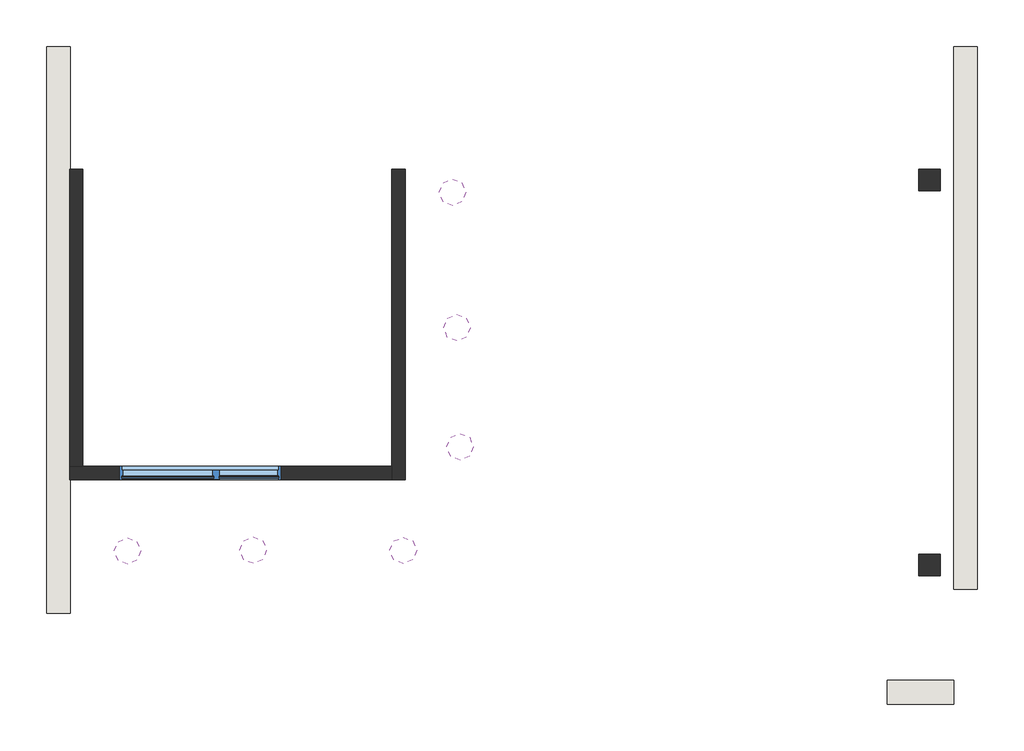
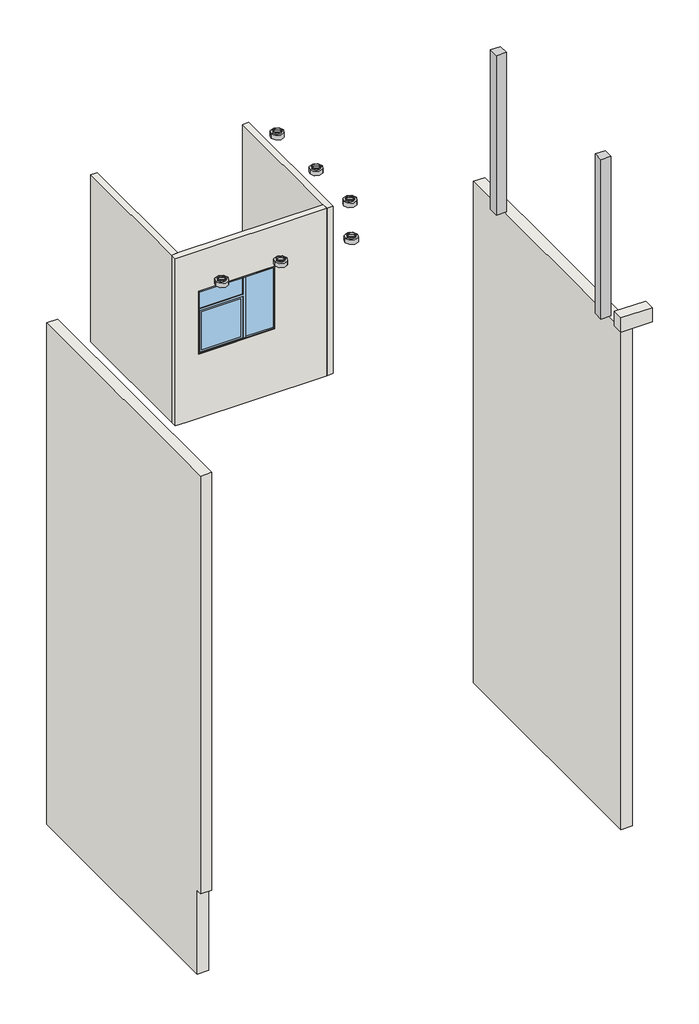
# One storey, incomplete: 6 light fixtures, 6 walls, 2 columns, 1 window.
"""IFC4 building model written with IfcOpenShell, lengths in millimetres."""

from ifc_helpers import new_model, si_unit, frame, origin, place, context, project, spatial, polyline, outline, extrude, faceted_brep, transform, mapped, element, save
from components import ceiling_light_flat_round_60w_120v_7c4c2a52, window_5c3f3b46

model = new_model("IFC4")

# Units and contexts
model_context = context("Model", 3, world=origin())
ifc_project = project(units=[si_unit("LENGTHUNIT", "METRE", prefix="MILLI")], contexts=[model_context])

# Site, building, storey
site = spatial("IfcSite", under=ifc_project)
building = spatial("IfcBuilding", under=site)
storey = spatial("IfcBuildingStorey", under=building, Elevation=13106.4)

# Columns
placement = place(None, origin())
element("IfcColumn", 1, ObjectType="Columns_Rectangular : 450x450mm", at=placement, inside=storey, context=model_context, shape_type="SweptSolid", body=[
    extrude(outline(polyline([(9092.5305046, -6363.9354899), (9092.5305046, -6567.1354899), (8889.3305046, -6567.1354899), (8889.3305046, -6363.9354899), (9092.5305046, -6363.9354899)])), frame((0.0, 0.0, 11887.2), z_axis=(0.0, 0.0, 1.0), x_axis=(1.0, 0.0, 0.0)), (0.0, 0.0, 1.0), 3418.8796875),
])
element("IfcColumn", 2, ObjectType="Columns_Rectangular : 450x450mm", at=placement, inside=storey, context=model_context, shape_type="SweptSolid", body=[
    extrude(outline(polyline([(9092.5305046, -2688.7252054), (9092.5305046, -2891.9252054), (8889.3305046, -2891.9252054), (8889.3305046, -2688.7252054), (9092.5305046, -2688.7252054)])), frame((0.0, 0.0, 11887.2), z_axis=(0.0, 0.0, 1.0), x_axis=(1.0, 0.0, 0.0)), (0.0, 0.0, 1.0), 3418.8796875),
])

# Light fixtures
ceiling_light_flat_round_60w_120v_shape = ceiling_light_flat_round_60w_120v_7c4c2a52(model_context)
element("IfcLightFixture", 3, ObjectType="Ceiling Light - Flat Round : 60W - 120V", at=placement, inside=storey, context=model_context, shape_type="MappedRepresentation", body=[
    mapped(ceiling_light_flat_round_60w_120v_shape, transform((1332.980672, -6332.2760393, 12828.6235673), x_axis=(1.0, 0.0, 0.0), y_axis=(0.0, 1.0, 0.0), z_axis=(0.0, 0.0, 1.0))),
])
element("IfcLightFixture", 4, ObjectType="Ceiling Light - Flat Round : 60W - 120V", at=placement, inside=storey, context=model_context, shape_type="MappedRepresentation", body=[
    mapped(ceiling_light_flat_round_60w_120v_shape, transform((2532.6708945, -6325.2433589, 12828.6235673), x_axis=(1.0, 0.0, 0.0), y_axis=(0.0, 1.0, 0.0), z_axis=(0.0, 0.0, 1.0))),
])
element("IfcLightFixture", 5, ObjectType="Ceiling Light - Flat Round : 60W - 120V", at=placement, inside=storey, context=model_context, shape_type="MappedRepresentation", body=[
    mapped(ceiling_light_flat_round_60w_120v_shape, transform((3965.0498814, -6327.1438327, 12828.6235673), x_axis=(1.0, 0.0, 0.0), y_axis=(0.0, 1.0, 0.0), z_axis=(0.0, 0.0, 1.0))),
])
element("IfcLightFixture", 6, ObjectType="Ceiling Light - Flat Round : 60W - 120V", at=placement, inside=storey, context=model_context, shape_type="MappedRepresentation", body=[
    mapped(ceiling_light_flat_round_60w_120v_shape, transform((4508.5834294, -5338.2131385, 12828.6235673), x_axis=(1.0, 0.0, 0.0), y_axis=(0.0, 1.0, 0.0), z_axis=(0.0, 0.0, 1.0))),
])
element("IfcLightFixture", 7, ObjectType="Ceiling Light - Flat Round : 60W - 120V", at=placement, inside=storey, context=model_context, shape_type="MappedRepresentation", body=[
    mapped(ceiling_light_flat_round_60w_120v_shape, transform((4477.7126249, -4200.8976487, 12828.6235673), x_axis=(1.0, 0.0, 0.0), y_axis=(0.0, 1.0, 0.0), z_axis=(0.0, 0.0, 1.0))),
])
element("IfcLightFixture", 8, ObjectType="Ceiling Light - Flat Round : 60W - 120V", at=placement, inside=storey, context=model_context, shape_type="MappedRepresentation", body=[
    mapped(ceiling_light_flat_round_60w_120v_shape, transform((4436.481358, -2908.1390402, 12828.6235673), x_axis=(1.0, 0.0, 0.0), y_axis=(0.0, 1.0, 0.0), z_axis=(0.0, 0.0, 1.0))),
])

# Walls
element("IfcWall", 9, ObjectType="5\"", at=placement, inside=storey, context=model_context, shape_type="Brep", body=[
    faceted_brep([(780.1132171, -5652.7354899, 15468.6), (780.1132171, -5652.7354899, 13106.4), (780.1132171, -5652.7354899, 11887.2), (1008.7132171, -5652.7354899, 11887.2), (3856.5941077, -5652.7354899, 11887.2), (3856.5941077, -5652.7354899, 15468.6), (1251.5536624, -5652.7354899, 14603.1645039), (2800.9536624, -5652.7354899, 14603.1645039), (2800.9536624, -5652.7354899, 13256.9645039), (1251.5536624, -5652.7354899, 13256.9645039), (780.1132171, -5525.7354899, 11887.2), (780.1132171, -5525.7354899, 15468.6), (907.1132171, -5525.7354899, 15468.6), (3856.5941077, -5525.7354899, 15468.6), (3856.5941077, -5525.7354899, 11887.2), (907.1132171, -5525.7354899, 11887.2), (1251.5536624, -5525.7354899, 14603.1645039), (1251.5536624, -5525.7354899, 13256.9645039), (2800.9536624, -5525.7354899, 13256.9645039), (2800.9536624, -5525.7354899, 14603.1645039)], [[[0, 1, 2, 3, 4, 5], [6, 7, 8, 9]], [[10, 11, 12, 13, 14, 15], [16, 17, 18, 19]], [[4, 3, 2, 10, 15, 14]], [[0, 5, 13, 12, 11]], [[0, 11, 10, 2, 1]], [[5, 4, 14, 13]], [[17, 16, 6, 9]], [[18, 17, 9, 8]], [[19, 18, 8, 7]], [[16, 19, 7, 6]]]),
])
element("IfcWall", 10, ObjectType="5\"", at=placement, inside=storey, context=model_context, shape_type="Brep", body=[
    faceted_brep([(3983.5941077, -5652.7354899, 11887.2), (3983.5941077, -2688.7252054, 11887.2), (3983.5941077, -2688.7252054, 15468.6), (3983.5941077, -5652.7354899, 15468.6), (3856.5941077, -5652.7354899, 11887.2), (3856.5941077, -5652.7354899, 15468.6), (3856.5941077, -5525.7354899, 15468.6), (3856.5941077, -2688.7252054, 15468.6), (3856.5941077, -2688.7252054, 11887.2), (3856.5941077, -5525.7354899, 11887.2)], [[[0, 1, 2, 3]], [[4, 5, 6, 7, 8, 9]], [[1, 0, 4, 9, 8]], [[2, 1, 8, 7]], [[3, 2, 7, 6, 5]], [[0, 3, 5, 4]]]),
])
element("IfcWall", 11, ObjectType="5\"", at=placement, inside=storey, context=model_context, shape_type="SweptSolid", body=[
    extrude(outline(polyline([(907.1132171, -2688.7252054), (907.1132171, -5525.7354899), (780.1132171, -5525.7354899), (780.1132171, -2688.7252054), (907.1132171, -2688.7252054)])), frame((0.0, 0.0, 11887.2), z_axis=(0.0, 0.0, 1.0), x_axis=(1.0, 0.0, 0.0)), (0.0, 0.0, 1.0), 3581.4),
])
element("IfcWall", 12, ObjectType="9\"", at=placement, inside=storey, context=model_context, shape_type="Brep", body=[
    faceted_brep([(788.1495839, -6811.7053244, 914.4), (788.1495839, -1515.8053244, 914.4), (788.1495839, -1515.8053244, 11658.6), (788.1495839, -6926.0053244, 11658.6), (788.1495839, -6926.0053244, 2706.0311436), (788.1495839, -6811.7053244, 2706.0311436), (788.1495839, -6811.7053244, 2089.1943747), (559.5495839, -6811.7053244, 914.4), (559.5495839, -6811.7053244, 2089.1943747), (559.5495839, -6811.7053244, 2706.0311436), (559.5495839, -6926.0053244, 2706.0311436), (559.5495839, -6926.0053244, 11658.6), (559.5495839, -1515.8053244, 11658.6), (559.5495839, -1515.8053244, 914.4)], [[[0, 1, 2, 3, 4, 5, 6]], [[7, 8, 9, 10, 11, 12, 13]], [[1, 0, 7, 13]], [[2, 1, 13, 12]], [[3, 2, 12, 11]], [[0, 6, 5, 9, 8, 7]], [[4, 10, 9, 5]], [[4, 3, 11, 10]]]),
])
element("IfcWall", 13, ObjectType="9\"", at=placement, inside=storey, context=model_context, shape_type="SweptSolid", body=[
    extrude(outline(polyline([(9448.1305046, -1515.8053244), (9448.1305046, -6697.4053244), (9219.5305046, -6697.4053244), (9219.5305046, -1515.8053244), (9448.1305046, -1515.8053244)])), frame((0.0, 0.0, 914.4), z_axis=(0.0, 0.0, 1.0), x_axis=(1.0, 0.0, 0.0)), (0.0, 0.0, 1.0), 10744.2),
])
element("IfcWall", 14, ObjectType="9\"", at=placement, inside=storey, context=model_context, shape_type="SweptSolid", body=[
    extrude(outline(polyline([(9219.5305046, -7793.6953528), (8587.7079602, -7793.6953528), (8587.7079602, -7565.0953528), (9219.5305046, -7565.0953528), (9219.5305046, -7793.6953528)])), frame((0.0, 0.0, 12458.7752496), z_axis=(0.0, 0.0, 1.0), x_axis=(1.0, 0.0, 0.0)), (0.0, 0.0, 1.0), 304.8),
])

# Window
window_shape = window_5c3f3b46(model_context)
element("IfcWindow", 15, ObjectType="Window-Casement-Double-Sidelight : 61\" x 53\"", at=placement, inside=storey, context=model_context, shape_type="MappedRepresentation", body=[
    mapped(window_shape, transform((2026.2536624, -5589.2354899, 12342.5645039), x_axis=(-1.0, 0.0, 0.0), y_axis=(0.0, -1.0, 0.0), z_axis=(0.0, 0.0, 1.0))),
])

save(model, "model.ifc")

# Revit data of these elements
# Type "Columns_Rectangular : 450x450mm"
#   Keynote = "G"
#   Depth = 0' - 8"
#   Offset Base = 0' - 0"
#   Offset Top = 0' - 0"
#   Width = 0' - 8"
#   Material = none
# Type "Ceiling Light - Flat Round : 60W - 120V"
#   Lamp = "A-19"
#   Assembly Code = "D5020220"
#   Wattage = 60 W
#   built-in parameter 1150110 = 1 (stored number, unit not read)
#   built-in parameter 1114217 = 1 (stored number, unit not read)
#   built-in parameter 1150109 = 1 (stored number, unit not read)
#   built-in parameter 1150113 = 1 (stored number, unit not read)
#   built-in parameter 1150115 = 1 (stored number, unit not read)
#   built-in parameter 1150105 = 272.155 (stored number, unit not read)
#   Light Source Symbol Size = 2' - 0"
#   built-in parameter 1150112 = 1 (stored number, unit not read)
#   built-in parameter 1150114 = 1 (stored number, unit not read)
#   built-in parameter 1150107 = 2800 (stored number, unit not read)
#   built-in parameter 1150106 = 2.72155 (stored number, unit not read)
#   Emit from Circle Diameter = 0' - 10"
#   built-in parameter 1150104 = 1.32387 (stored number, unit not read)
#   Ballast Voltage = 120 V
#   built-in parameter 1114218 = 1 (stored number, unit not read)
#   built-in parameter 1150133 = 10 (stored number, unit not read)
#   Lumens = 855 lm
#   Apparent Load = 60 VA
#   built-in parameter 1150134 = 4
#   built-in parameter 1150137 = 1
#   Color Filter = 16777215
#   built-in parameter 1140040 [instance default] = 1
#   Ballast Number of Poles = 1
#   Light Box Material = Steel, Paint Finish, Dark Gray, Matte
#   Diffuser Material = Glass, White, High Luminance
#   Wattage Comments = ""
#   Emit Shape Visible in Rendering = no
#   Dimming Lamp Color Temperature Shift = (empty or 0)
#   Default Elevation = 0
# Type "5\""
#   Keynote = "F10"
#   Layers, outside or top first: 0' - 5" "Concrete" (function 1)
# Type "9\""
#   Keynote = "F10"
#   Layers, outside or top first: 0' - 9" "Concrete" (function 1)
# Type "Window-Casement-Double-Sidelight : 61\" x 53\""
#   Type Mark = "55"
#   Fire Rating = "0.5h"
#   Assembly Code = "B2020100"
#   Analytic Construction = "Double glazing - domestic"
#   Window Inset [instance default] = 0' - 0 5/8"
#   Wall Thickness [instance default] = 0' - 6"
#   Visual Light Transmittance = 0.81
#   Transom Height Ratio = 0.3
#   Transom Height = 1' - 3.9"
#   Thermal Resistance (R) = 0.319569 (m²·K)/W
#   Solar Heat Gain Coefficient = 0.76
#   Side Width = 2' - 0.4"
#   Rough Width = 5' - 1 1/2"
#   Rough Height = 4' - 5 1/2"
#   Opening Window Width = 3' - 0.6"
#   Opening Window Height = 3' - 1.1"
#   Heat Transfer Coefficient (U) = 3.12929 W/(m²·K)
#   Height = 4' - 5"
#   Frame Gap 3 [instance default] = 0' - 1 83/128"
#   Frame Gap 2 [instance default] = 0' - 0 5/8"
#   Frame Gap 1 = 0' - 1 51/128"
#   Default Sill Height = 3' - 0"
#   Width = 5' - 1"
#   Frame Material = Metal - Aluminum
#   Glass Panel Material = Glass
#   Wall Closure = (empty or 0)
# Elements 1, 2 (IfcColumn, "Columns_Rectangular : 450x450mm")
#   Phase Created = New Construction
#   Materials on its faces: "Gypsum Wall Board"
# Element 3 (IfcLightFixture, "Ceiling Light - Flat Round : 60W - 120V")
#   Mark = "1"
#   built-in parameter 1140040 = 1
#   Phase Created = New Construction
#   Materials on its faces: "Glass, White, High Luminance", "Steel, Paint Finish, Dark Gray, Matte"
# Element 4 (IfcLightFixture, "Ceiling Light - Flat Round : 60W - 120V")
#   Mark = "2"
#   built-in parameter 1140040 = 1
#   Phase Created = New Construction
#   Materials on its faces: "Glass, White, High Luminance", "Steel, Paint Finish, Dark Gray, Matte"
# Element 5 (IfcLightFixture, "Ceiling Light - Flat Round : 60W - 120V")
#   Mark = "3"
#   built-in parameter 1140040 = 1
#   Phase Created = New Construction
#   Materials on its faces: "Glass, White, High Luminance", "Steel, Paint Finish, Dark Gray, Matte"
# Element 6 (IfcLightFixture, "Ceiling Light - Flat Round : 60W - 120V")
#   Mark = "4"
#   built-in parameter 1140040 = 1
#   Phase Created = New Construction
#   Materials on its faces: "Glass, White, High Luminance", "Steel, Paint Finish, Dark Gray, Matte"
# Element 7 (IfcLightFixture, "Ceiling Light - Flat Round : 60W - 120V")
#   Mark = "5"
#   built-in parameter 1140040 = 1
#   Phase Created = New Construction
#   Materials on its faces: "Glass, White, High Luminance", "Steel, Paint Finish, Dark Gray, Matte"
# Element 8 (IfcLightFixture, "Ceiling Light - Flat Round : 60W - 120V")
#   Mark = "6"
#   built-in parameter 1140040 = 1
#   Phase Created = New Construction
#   Materials on its faces: "Glass, White, High Luminance", "Steel, Paint Finish, Dark Gray, Matte"
# Elements 9, 11 (IfcWall, "5\"")
#   built-in parameter 1001111 = -4' - 0"
#   Top Offset = 0' - 0"
#   Base Offset = -4' - 0"
#   wall height = 11' - 9"
#   Phase Created = New Construction
#   Materials on its faces: "Concrete", "Blue"
# Element 10 (IfcWall, "5\"")
#   built-in parameter 1001111 = -4' - 0"
#   Top Offset = 0' - 0"
#   Base Offset = -4' - 0"
#   wall height = 11' - 9"
#   Phase Created = New Construction
#   Materials on its faces: "Concrete", "Clad - White", "Blue"
# Elements 12, 13 (IfcWall, "9\"")
#   built-in parameter 1001111 = -40' - 0"
#   Top Offset = -12' - 6"
#   Base Offset = -40' - 0"
#   wall height = 35' - 3"
#   Phase Created = New Construction
#   Materials on its faces: "Concrete", "Gypsum Wall Board"
# Element 14 (IfcWall, "9\"")
#   built-in parameter 1001111 = -2' - 1.49704"
#   Top Offset = -7' - 9"
#   Base Offset = -2' - 1.49704"
#   Unconnected Height = 1' - 0"
#   wall height = 1' - 0"
#   Phase Created = New Construction
#   Materials on its faces: "Concrete", "Earth"
# Element 15 (IfcWindow, "Window-Casement-Double-Sidelight : 61\" x 53\"")
#   Mark = "7"
#   Window Inset = 0' - 0 5/8"
#   Frame Gap 3 = 0' - 1 83/128"
#   Frame Gap 2 = 0' - 0 5/8"
#   Phase Created = New Construction
#   Materials on its faces: "Metal - Aluminum", "Glass"
# Materials
#   "Steel, Paint Finish, Dark Gray, Matte": class "Metal", colour RGB 98 98 98, transparency 0, Description = "Steel, paint finish, dark gray, matte", Cost = 0
#   "Glass, White, High Luminance": class "Glass", colour RGB 249 250 249, transparency 0.8, Description = "physical material", Cost = 0
#   "Concrete": class "Concrete", colour RGB 120 120 120, transparency 0, Description = "Portland Cement Concrete", Cost = 0
#   "Metal - Aluminum": class "Metal", colour RGB 247 247 247, transparency 0
#   "Glass": class "Glass", colour RGB 0 128 192, transparency 0.9, Description = "Soda Lime Glass", Cost = 0
#   "Gypsum Wall Board": class "Generic", colour RGB 249 249 249, transparency 0, Description = "Gypsum Wall Board", Cost = 0
#   "Blue": class "Generic", colour RGB 0 43 85, transparency 0, Cost = 0
#   "Clad - White": class "Wood", colour RGB 242 242 238, transparency 0, Cost = 0
#   "Earth": class "Generic", colour RGB 97 75 62, transparency 0, Description = "Soil", Cost = 0
